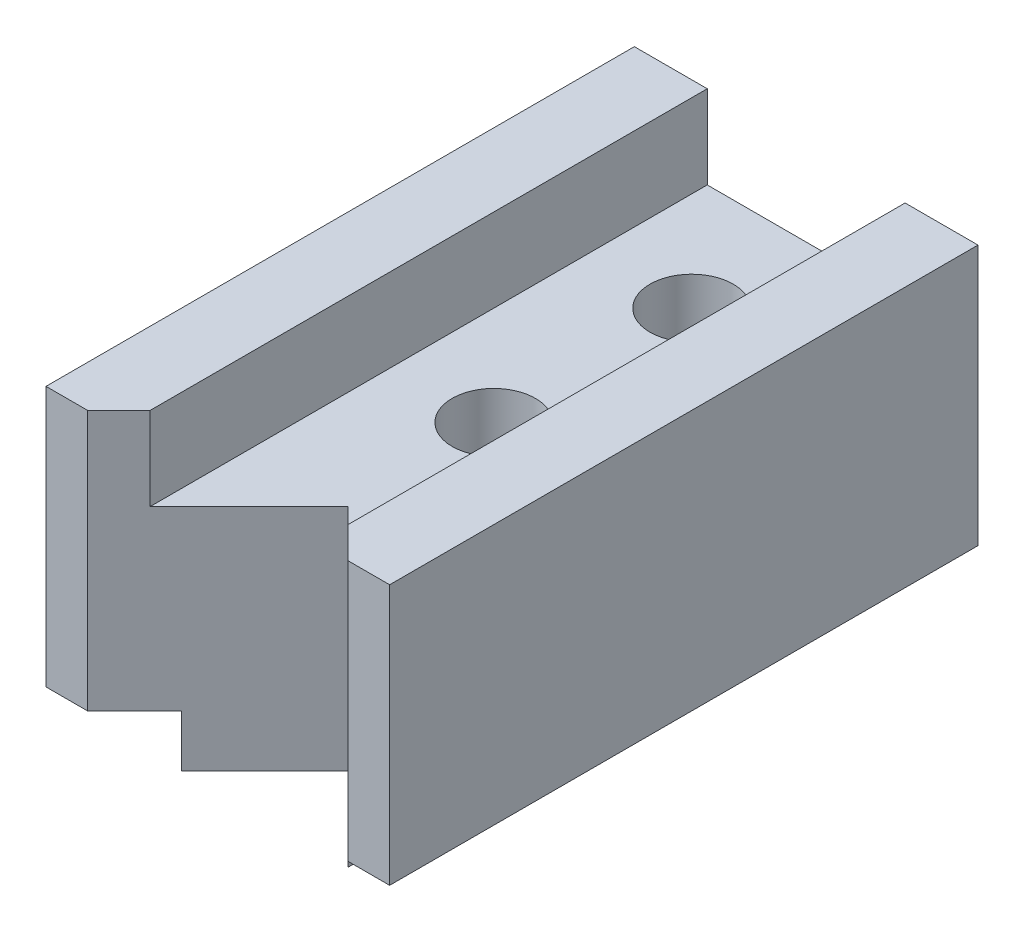
ISO-10303-21;
HEADER;
FILE_DESCRIPTION(('STEP AP214'),'2;1');
FILE_NAME('part.step','',(''),(''),'','','');
FILE_SCHEMA(('AUTOMOTIVE_DESIGN { 1 0 10303 214 1 1 1 1 }'));
ENDSEC;
DATA;
#1=APPLICATION_CONTEXT('core data for automotive mechanical design processes');
#2=APPLICATION_PROTOCOL_DEFINITION('international standard','automotive_design',2000,#1);
#3=PRODUCT_CONTEXT('',#1,'mechanical');
#4=PRODUCT('Part','Part','',(#3));
#5=PRODUCT_RELATED_PRODUCT_CATEGORY('part','',(#4));
#6=PRODUCT_DEFINITION_FORMATION('','',#4);
#7=PRODUCT_DEFINITION_CONTEXT('part definition',#1,'design');
#8=PRODUCT_DEFINITION('design','',#6,#7);
#9=PRODUCT_DEFINITION_SHAPE('','',#8);
#10=(LENGTH_UNIT() NAMED_UNIT(*) SI_UNIT(.MILLI.,.METRE.));
#11=(NAMED_UNIT(*) PLANE_ANGLE_UNIT() SI_UNIT($,.RADIAN.));
#12=(NAMED_UNIT(*) SI_UNIT($,.STERADIAN.) SOLID_ANGLE_UNIT());
#13=UNCERTAINTY_MEASURE_WITH_UNIT(LENGTH_MEASURE(1.E-05),#10,'distance_accuracy_value','');
#14=(GEOMETRIC_REPRESENTATION_CONTEXT(3) GLOBAL_UNCERTAINTY_ASSIGNED_CONTEXT((#13)) GLOBAL_UNIT_ASSIGNED_CONTEXT((#10,
#11,#12)) REPRESENTATION_CONTEXT('',''));
#15=CARTESIAN_POINT('',(0.,0.,0.));
#16=DIRECTION('',(0.,0.,1.));
#17=DIRECTION('',(1.,0.,0.));
#18=AXIS2_PLACEMENT_3D('',#15,#16,#17);
#19=CARTESIAN_POINT('',(0.,0.,56.5));
#20=DIRECTION('',(0.,0.,-1.));
#21=DIRECTION('',(-1.,0.,0.));
#22=AXIS2_PLACEMENT_3D('',#19,#20,#21);
#23=PLANE('',#22);
#24=DIRECTION('',(0.,-1.,0.));
#25=VECTOR('',#24,1.);
#26=CARTESIAN_POINT('',(8.00000000000009,179.9522506111,56.5));
#27=LINE('',#26,#25);
#28=CARTESIAN_POINT('',(8.00000000000009,50.,56.5));
#29=VERTEX_POINT('',#28);
#30=CARTESIAN_POINT('',(8.00000000000009,0.,56.5));
#31=VERTEX_POINT('',#30);
#32=EDGE_CURVE('E11',#29,#31,#27,.T.);
#33=ORIENTED_EDGE('',*,*,#32,.F.);
#34=DIRECTION('',(-1.,0.,0.));
#35=VECTOR('',#34,1.);
#36=CARTESIAN_POINT('',(0.,50.,56.5));
#37=LINE('',#36,#35);
#38=CARTESIAN_POINT('',(0.,50.,56.5));
#39=VERTEX_POINT('',#38);
#40=EDGE_CURVE('E180',#29,#39,#37,.T.);
#41=ORIENTED_EDGE('',*,*,#40,.T.);
#42=DIRECTION('',(0.,-1.,0.));
#43=VECTOR('',#42,1.);
#44=CARTESIAN_POINT('',(0.,0.,56.5));
#45=LINE('',#44,#43);
#46=CARTESIAN_POINT('',(0.,0.,56.5));
#47=VERTEX_POINT('',#46);
#48=EDGE_CURVE('E64',#39,#47,#45,.T.);
#49=ORIENTED_EDGE('',*,*,#48,.T.);
#50=DIRECTION('',(1.,0.,0.));
#51=VECTOR('',#50,1.);
#52=CARTESIAN_POINT('',(17.,0.,56.5));
#53=LINE('',#52,#51);
#54=EDGE_CURVE('E220',#47,#31,#53,.T.);
#55=ORIENTED_EDGE('',*,*,#54,.T.);
#56=EDGE_LOOP('',(#33,#41,#49,#55));
#57=FACE_BOUND('',#56,.T.);
#58=ADVANCED_FACE('F39',(#57),#23,.F.);
#59=CARTESIAN_POINT('',(17.,0.,56.5));
#60=DIRECTION('',(0.,1.,0.));
#61=DIRECTION('',(0.,0.,1.));
#62=AXIS2_PLACEMENT_3D('',#59,#60,#61);
#63=PLANE('',#62);
#64=DIRECTION('',(0.,0.,-1.));
#65=VECTOR('',#64,1.);
#66=CARTESIAN_POINT('',(17.,0.,56.5));
#67=LINE('',#66,#65);
#68=CARTESIAN_POINT('',(17.,0.,47.5000000000001));
#69=VERTEX_POINT('',#68);
#70=CARTESIAN_POINT('',(17.,0.,-56.5));
#71=VERTEX_POINT('',#70);
#72=EDGE_CURVE('E43',#69,#71,#67,.T.);
#73=ORIENTED_EDGE('',*,*,#72,.F.);
#74=DIRECTION('',(-0.707106781186546,0.,0.707106781186549));
#75=VECTOR('',#74,1.);
#76=CARTESIAN_POINT('',(12.5,0.,52.));
#77=LINE('',#76,#75);
#78=EDGE_CURVE('E419',#69,#31,#77,.T.);
#79=ORIENTED_EDGE('',*,*,#78,.T.);
#80=ORIENTED_EDGE('',*,*,#54,.F.);
#81=DIRECTION('',(0.,0.,-1.));
#82=VECTOR('',#81,1.);
#83=CARTESIAN_POINT('',(0.,0.,56.5));
#84=LINE('',#83,#82);
#85=CARTESIAN_POINT('',(0.,0.,-56.5));
#86=VERTEX_POINT('',#85);
#87=EDGE_CURVE('E183',#47,#86,#84,.T.);
#88=ORIENTED_EDGE('',*,*,#87,.T.);
#89=DIRECTION('',(1.,0.,0.));
#90=VECTOR('',#89,1.);
#91=CARTESIAN_POINT('',(17.,0.,-56.5));
#92=LINE('',#91,#90);
#93=EDGE_CURVE('E186',#86,#71,#92,.T.);
#94=ORIENTED_EDGE('',*,*,#93,.T.);
#95=EDGE_LOOP('',(#73,#79,#80,#88,#94));
#96=FACE_BOUND('',#95,.T.);
#97=ADVANCED_FACE('F41',(#96),#63,.F.);
#98=CARTESIAN_POINT('',(17.,-10.,56.5));
#99=DIRECTION('',(1.,0.,0.));
#100=DIRECTION('',(0.,0.,-1.));
#101=AXIS2_PLACEMENT_3D('',#98,#99,#100);
#102=PLANE('',#101);
#103=DIRECTION('',(0.,0.,-1.));
#104=VECTOR('',#103,1.);
#105=CARTESIAN_POINT('',(17.,-10.,56.5));
#106=LINE('',#105,#104);
#107=CARTESIAN_POINT('',(17.,-10.,47.5000000000001));
#108=VERTEX_POINT('',#107);
#109=CARTESIAN_POINT('',(17.,-10.,-56.5));
#110=VERTEX_POINT('',#109);
#111=EDGE_CURVE('E237',#108,#110,#106,.T.);
#112=ORIENTED_EDGE('',*,*,#111,.F.);
#113=DIRECTION('',(0.,1.,0.));
#114=VECTOR('',#113,1.);
#115=CARTESIAN_POINT('',(17.,-10.,47.5000000000001));
#116=LINE('',#115,#114);
#117=EDGE_CURVE('E249',#108,#69,#116,.T.);
#118=ORIENTED_EDGE('',*,*,#117,.T.);
#119=ORIENTED_EDGE('',*,*,#72,.T.);
#120=DIRECTION('',(0.,-1.,0.));
#121=VECTOR('',#120,1.);
#122=CARTESIAN_POINT('',(17.,-10.,-56.5));
#123=LINE('',#122,#121);
#124=EDGE_CURVE('E188',#71,#110,#123,.T.);
#125=ORIENTED_EDGE('',*,*,#124,.T.);
#126=EDGE_LOOP('',(#112,#118,#119,#125));
#127=FACE_BOUND('',#126,.T.);
#128=ADVANCED_FACE('F243',(#127),#102,.F.);
#129=CARTESIAN_POINT('',(49.,-10.,56.5));
#130=DIRECTION('',(0.,1.,0.));
#131=DIRECTION('',(-1.,0.,0.));
#132=AXIS2_PLACEMENT_3D('',#129,#130,#131);
#133=PLANE('',#132);
#134=CARTESIAN_POINT('',(33.,-10.,-34.5));
#135=DIRECTION('',(0.,1.,0.));
#136=DIRECTION('',(0.,0.,1.));
#137=AXIS2_PLACEMENT_3D('',#134,#135,#136);
#138=CIRCLE('',#137,8.);
#139=CARTESIAN_POINT('',(33.,-10.,-26.5));
#140=VERTEX_POINT('',#139);
#141=EDGE_CURVE('E189',#140,#140,#138,.T.);
#142=ORIENTED_EDGE('',*,*,#141,.T.);
#143=EDGE_LOOP('',(#142));
#144=FACE_BOUND('',#143,.T.);
#145=CARTESIAN_POINT('',(33.,-10.,3.5));
#146=DIRECTION('',(0.,1.,0.));
#147=DIRECTION('',(0.,0.,1.));
#148=AXIS2_PLACEMENT_3D('',#145,#146,#147);
#149=CIRCLE('',#148,8.);
#150=CARTESIAN_POINT('',(33.,-10.,11.5));
#151=VERTEX_POINT('',#150);
#152=EDGE_CURVE('E424',#151,#151,#149,.T.);
#153=ORIENTED_EDGE('',*,*,#152,.T.);
#154=EDGE_LOOP('',(#153));
#155=FACE_BOUND('',#154,.T.);
#156=DIRECTION('',(-0.707106781186547,0.,-0.707106781186549));
#157=VECTOR('',#156,1.);
#158=CARTESIAN_POINT('',(53.5,-10.,52.));
#159=LINE('',#158,#157);
#160=CARTESIAN_POINT('',(49.,-10.,47.5));
#161=VERTEX_POINT('',#160);
#162=CARTESIAN_POINT('',(33.,-10.,31.5));
#163=VERTEX_POINT('',#162);
#164=EDGE_CURVE('E287',#161,#163,#159,.T.);
#165=ORIENTED_EDGE('',*,*,#164,.T.);
#166=DIRECTION('',(-0.707106781186546,0.,0.707106781186549));
#167=VECTOR('',#166,1.);
#168=CARTESIAN_POINT('',(28.5,-10.,36.));
#169=LINE('',#168,#167);
#170=EDGE_CURVE('E426',#163,#108,#169,.T.);
#171=ORIENTED_EDGE('',*,*,#170,.T.);
#172=ORIENTED_EDGE('',*,*,#111,.T.);
#173=DIRECTION('',(1.,0.,0.));
#174=VECTOR('',#173,1.);
#175=CARTESIAN_POINT('',(49.,-10.,-56.5));
#176=LINE('',#175,#174);
#177=CARTESIAN_POINT('',(49.,-10.,-56.5));
#178=VERTEX_POINT('',#177);
#179=EDGE_CURVE('E195',#110,#178,#176,.T.);
#180=ORIENTED_EDGE('',*,*,#179,.T.);
#181=DIRECTION('',(0.,0.,-1.));
#182=VECTOR('',#181,1.);
#183=CARTESIAN_POINT('',(49.,-10.,56.5));
#184=LINE('',#183,#182);
#185=EDGE_CURVE('E232',#161,#178,#184,.T.);
#186=ORIENTED_EDGE('',*,*,#185,.F.);
#187=EDGE_LOOP('',(#165,#171,#172,#180,#186));
#188=FACE_BOUND('',#187,.T.);
#189=ADVANCED_FACE('F288',(#144,#155,#188),#133,.F.);
#190=CARTESIAN_POINT('',(49.,0.,56.5));
#191=DIRECTION('',(-1.,0.,0.));
#192=DIRECTION('',(0.,0.,1.));
#193=AXIS2_PLACEMENT_3D('',#190,#191,#192);
#194=PLANE('',#193);
#195=DIRECTION('',(0.,0.,-1.));
#196=VECTOR('',#195,1.);
#197=CARTESIAN_POINT('',(49.,0.,56.5));
#198=LINE('',#197,#196);
#199=CARTESIAN_POINT('',(49.,0.,47.5));
#200=VERTEX_POINT('',#199);
#201=CARTESIAN_POINT('',(49.,0.,-56.5));
#202=VERTEX_POINT('',#201);
#203=EDGE_CURVE('E235',#200,#202,#198,.T.);
#204=ORIENTED_EDGE('',*,*,#203,.F.);
#205=DIRECTION('',(0.,-1.,0.));
#206=VECTOR('',#205,1.);
#207=CARTESIAN_POINT('',(49.,0.,47.5));
#208=LINE('',#207,#206);
#209=EDGE_CURVE('E286',#200,#161,#208,.T.);
#210=ORIENTED_EDGE('',*,*,#209,.T.);
#211=ORIENTED_EDGE('',*,*,#185,.T.);
#212=DIRECTION('',(0.,1.,0.));
#213=VECTOR('',#212,1.);
#214=CARTESIAN_POINT('',(49.,0.,-56.5));
#215=LINE('',#214,#213);
#216=EDGE_CURVE('E198',#178,#202,#215,.T.);
#217=ORIENTED_EDGE('',*,*,#216,.T.);
#218=EDGE_LOOP('',(#204,#210,#211,#217));
#219=FACE_BOUND('',#218,.T.);
#220=ADVANCED_FACE('F284',(#219),#194,.F.);
#221=CARTESIAN_POINT('',(66.,0.,56.5));
#222=DIRECTION('',(0.,1.,0.));
#223=DIRECTION('',(0.,0.,1.));
#224=AXIS2_PLACEMENT_3D('',#221,#222,#223);
#225=PLANE('',#224);
#226=DIRECTION('',(1.,0.,0.));
#227=VECTOR('',#226,1.);
#228=CARTESIAN_POINT('',(66.,0.,56.5));
#229=LINE('',#228,#227);
#230=CARTESIAN_POINT('',(57.9999999999999,0.,56.5));
#231=VERTEX_POINT('',#230);
#232=CARTESIAN_POINT('',(66.,0.,56.5));
#233=VERTEX_POINT('',#232);
#234=EDGE_CURVE('E117',#231,#233,#229,.T.);
#235=ORIENTED_EDGE('',*,*,#234,.F.);
#236=DIRECTION('',(-0.707106781186547,0.,-0.707106781186549));
#237=VECTOR('',#236,1.);
#238=CARTESIAN_POINT('',(62.,0.,60.5));
#239=LINE('',#238,#237);
#240=EDGE_CURVE('E161',#231,#200,#239,.T.);
#241=ORIENTED_EDGE('',*,*,#240,.T.);
#242=ORIENTED_EDGE('',*,*,#203,.T.);
#243=DIRECTION('',(1.,0.,0.));
#244=VECTOR('',#243,1.);
#245=CARTESIAN_POINT('',(66.,0.,-56.5));
#246=LINE('',#245,#244);
#247=CARTESIAN_POINT('',(66.,0.,-56.5));
#248=VERTEX_POINT('',#247);
#249=EDGE_CURVE('E200',#202,#248,#246,.T.);
#250=ORIENTED_EDGE('',*,*,#249,.T.);
#251=DIRECTION('',(0.,0.,-1.));
#252=VECTOR('',#251,1.);
#253=CARTESIAN_POINT('',(66.,0.,56.5));
#254=LINE('',#253,#252);
#255=EDGE_CURVE('E229',#233,#248,#254,.T.);
#256=ORIENTED_EDGE('',*,*,#255,.F.);
#257=EDGE_LOOP('',(#235,#241,#242,#250,#256));
#258=FACE_BOUND('',#257,.T.);
#259=ADVANCED_FACE('F281',(#258),#225,.F.);
#260=CARTESIAN_POINT('',(66.,50.,56.5));
#261=DIRECTION('',(-1.,0.,0.));
#262=DIRECTION('',(0.,0.,1.));
#263=AXIS2_PLACEMENT_3D('',#260,#261,#262);
#264=PLANE('',#263);
#265=DIRECTION('',(0.,1.,0.));
#266=VECTOR('',#265,1.);
#267=CARTESIAN_POINT('',(66.,50.,-56.5));
#268=LINE('',#267,#266);
#269=CARTESIAN_POINT('',(66.,50.,-56.5));
#270=VERTEX_POINT('',#269);
#271=EDGE_CURVE('E203',#248,#270,#268,.T.);
#272=ORIENTED_EDGE('',*,*,#271,.T.);
#273=DIRECTION('',(0.,0.,-1.));
#274=VECTOR('',#273,1.);
#275=CARTESIAN_POINT('',(66.,50.,56.5));
#276=LINE('',#275,#274);
#277=CARTESIAN_POINT('',(66.,50.,56.5));
#278=VERTEX_POINT('',#277);
#279=EDGE_CURVE('E227',#278,#270,#276,.T.);
#280=ORIENTED_EDGE('',*,*,#279,.F.);
#281=DIRECTION('',(0.,1.,0.));
#282=VECTOR('',#281,1.);
#283=CARTESIAN_POINT('',(66.,50.,56.5));
#284=LINE('',#283,#282);
#285=EDGE_CURVE('E179',#233,#278,#284,.T.);
#286=ORIENTED_EDGE('',*,*,#285,.F.);
#287=ORIENTED_EDGE('',*,*,#255,.T.);
#288=EDGE_LOOP('',(#272,#280,#286,#287));
#289=FACE_BOUND('',#288,.T.);
#290=ADVANCED_FACE('F279',(#289),#264,.F.);
#291=CARTESIAN_POINT('',(52.,50.,56.5));
#292=DIRECTION('',(0.,-1.,0.));
#293=DIRECTION('',(0.,0.,-1.));
#294=AXIS2_PLACEMENT_3D('',#291,#292,#293);
#295=PLANE('',#294);
#296=DIRECTION('',(0.,0.,-1.));
#297=VECTOR('',#296,1.);
#298=CARTESIAN_POINT('',(52.,50.,56.5));
#299=LINE('',#298,#297);
#300=CARTESIAN_POINT('',(52.,50.,50.5000000000001));
#301=VERTEX_POINT('',#300);
#302=CARTESIAN_POINT('',(52.,50.,-56.5));
#303=VERTEX_POINT('',#302);
#304=EDGE_CURVE('E171',#301,#303,#299,.T.);
#305=ORIENTED_EDGE('',*,*,#304,.F.);
#306=DIRECTION('',(0.707106781186547,0.,0.707106781186549));
#307=VECTOR('',#306,1.);
#308=CARTESIAN_POINT('',(55.,50.,53.5));
#309=LINE('',#308,#307);
#310=CARTESIAN_POINT('',(57.9999999999999,50.,56.5));
#311=VERTEX_POINT('',#310);
#312=EDGE_CURVE('E158',#301,#311,#309,.T.);
#313=ORIENTED_EDGE('',*,*,#312,.T.);
#314=DIRECTION('',(-1.,0.,0.));
#315=VECTOR('',#314,1.);
#316=CARTESIAN_POINT('',(52.,50.,56.5));
#317=LINE('',#316,#315);
#318=EDGE_CURVE('E166',#278,#311,#317,.T.);
#319=ORIENTED_EDGE('',*,*,#318,.F.);
#320=ORIENTED_EDGE('',*,*,#279,.T.);
#321=DIRECTION('',(-1.,0.,0.));
#322=VECTOR('',#321,1.);
#323=CARTESIAN_POINT('',(52.,50.,-56.5));
#324=LINE('',#323,#322);
#325=EDGE_CURVE('E201',#270,#303,#324,.T.);
#326=ORIENTED_EDGE('',*,*,#325,.T.);
#327=EDGE_LOOP('',(#305,#313,#319,#320,#326));
#328=FACE_BOUND('',#327,.T.);
#329=ADVANCED_FACE('F170',(#328),#295,.F.);
#330=CARTESIAN_POINT('',(52.,34.,56.5));
#331=DIRECTION('',(1.,0.,0.));
#332=DIRECTION('',(0.,0.,-1.));
#333=AXIS2_PLACEMENT_3D('',#330,#331,#332);
#334=PLANE('',#333);
#335=DIRECTION('',(0.,0.,-1.));
#336=VECTOR('',#335,1.);
#337=CARTESIAN_POINT('',(52.,34.,56.5));
#338=LINE('',#337,#336);
#339=CARTESIAN_POINT('',(52.,34.,50.5));
#340=VERTEX_POINT('',#339);
#341=CARTESIAN_POINT('',(52.,34.,-56.5));
#342=VERTEX_POINT('',#341);
#343=EDGE_CURVE('E223',#340,#342,#338,.T.);
#344=ORIENTED_EDGE('',*,*,#343,.F.);
#345=DIRECTION('',(0.,1.,0.));
#346=VECTOR('',#345,1.);
#347=CARTESIAN_POINT('',(52.,34.,50.5000000000001));
#348=LINE('',#347,#346);
#349=EDGE_CURVE('E175',#340,#301,#348,.T.);
#350=ORIENTED_EDGE('',*,*,#349,.T.);
#351=ORIENTED_EDGE('',*,*,#304,.T.);
#352=DIRECTION('',(0.,-1.,0.));
#353=VECTOR('',#352,1.);
#354=CARTESIAN_POINT('',(52.,34.,-56.5));
#355=LINE('',#354,#353);
#356=EDGE_CURVE('E202',#303,#342,#355,.T.);
#357=ORIENTED_EDGE('',*,*,#356,.T.);
#358=EDGE_LOOP('',(#344,#350,#351,#357));
#359=FACE_BOUND('',#358,.T.);
#360=ADVANCED_FACE('F277',(#359),#334,.F.);
#361=CARTESIAN_POINT('',(14.,34.,56.5));
#362=DIRECTION('',(0.,-1.,0.));
#363=DIRECTION('',(0.,0.,-1.));
#364=AXIS2_PLACEMENT_3D('',#361,#362,#363);
#365=PLANE('',#364);
#366=CARTESIAN_POINT('',(33.,34.,-34.5));
#367=DIRECTION('',(0.,1.,0.));
#368=DIRECTION('',(0.,0.,1.));
#369=AXIS2_PLACEMENT_3D('',#366,#367,#368);
#370=CIRCLE('',#369,8.);
#371=CARTESIAN_POINT('',(33.,34.,-26.5));
#372=VERTEX_POINT('',#371);
#373=EDGE_CURVE('E431',#372,#372,#370,.T.);
#374=ORIENTED_EDGE('',*,*,#373,.F.);
#375=EDGE_LOOP('',(#374));
#376=FACE_BOUND('',#375,.T.);
#377=CARTESIAN_POINT('',(33.,34.,3.5));
#378=DIRECTION('',(0.,1.,0.));
#379=DIRECTION('',(0.,0.,1.));
#380=AXIS2_PLACEMENT_3D('',#377,#378,#379);
#381=CIRCLE('',#380,8.);
#382=CARTESIAN_POINT('',(33.,34.,11.5));
#383=VERTEX_POINT('',#382);
#384=EDGE_CURVE('E423',#383,#383,#381,.T.);
#385=ORIENTED_EDGE('',*,*,#384,.F.);
#386=EDGE_LOOP('',(#385));
#387=FACE_BOUND('',#386,.T.);
#388=DIRECTION('',(0.,0.,-1.));
#389=VECTOR('',#388,1.);
#390=CARTESIAN_POINT('',(14.,34.,56.5));
#391=LINE('',#390,#389);
#392=CARTESIAN_POINT('',(14.,34.,50.5000000000001));
#393=VERTEX_POINT('',#392);
#394=CARTESIAN_POINT('',(14.,34.,-56.5));
#395=VERTEX_POINT('',#394);
#396=EDGE_CURVE('E224',#393,#395,#391,.T.);
#397=ORIENTED_EDGE('',*,*,#396,.F.);
#398=DIRECTION('',(0.707106781186546,0.,-0.707106781186549));
#399=VECTOR('',#398,1.);
#400=CARTESIAN_POINT('',(11.,34.,53.5));
#401=LINE('',#400,#399);
#402=CARTESIAN_POINT('',(33.,34.,31.5));
#403=VERTEX_POINT('',#402);
#404=EDGE_CURVE('E441',#393,#403,#401,.T.);
#405=ORIENTED_EDGE('',*,*,#404,.T.);
#406=DIRECTION('',(0.707106781186547,0.,0.707106781186549));
#407=VECTOR('',#406,1.);
#408=CARTESIAN_POINT('',(36.,34.,34.5));
#409=LINE('',#408,#407);
#410=EDGE_CURVE('E451',#403,#340,#409,.T.);
#411=ORIENTED_EDGE('',*,*,#410,.T.);
#412=ORIENTED_EDGE('',*,*,#343,.T.);
#413=DIRECTION('',(-1.,0.,0.));
#414=VECTOR('',#413,1.);
#415=CARTESIAN_POINT('',(14.,34.,-56.5));
#416=LINE('',#415,#414);
#417=EDGE_CURVE('E208',#342,#395,#416,.T.);
#418=ORIENTED_EDGE('',*,*,#417,.T.);
#419=EDGE_LOOP('',(#397,#405,#411,#412,#418));
#420=FACE_BOUND('',#419,.T.);
#421=ADVANCED_FACE('F267',(#376,#387,#420),#365,.F.);
#422=CARTESIAN_POINT('',(14.,50.,56.5));
#423=DIRECTION('',(-1.,0.,0.));
#424=DIRECTION('',(0.,-1.,0.));
#425=AXIS2_PLACEMENT_3D('',#422,#423,#424);
#426=PLANE('',#425);
#427=DIRECTION('',(0.,0.,-1.));
#428=VECTOR('',#427,1.);
#429=CARTESIAN_POINT('',(14.,50.,56.5));
#430=LINE('',#429,#428);
#431=CARTESIAN_POINT('',(14.,50.,50.5000000000001));
#432=VERTEX_POINT('',#431);
#433=CARTESIAN_POINT('',(14.,50.,-56.5));
#434=VERTEX_POINT('',#433);
#435=EDGE_CURVE('E222',#432,#434,#430,.T.);
#436=ORIENTED_EDGE('',*,*,#435,.F.);
#437=DIRECTION('',(0.,-1.,0.));
#438=VECTOR('',#437,1.);
#439=CARTESIAN_POINT('',(14.,50.,50.5000000000001));
#440=LINE('',#439,#438);
#441=EDGE_CURVE('E57',#432,#393,#440,.T.);
#442=ORIENTED_EDGE('',*,*,#441,.T.);
#443=ORIENTED_EDGE('',*,*,#396,.T.);
#444=DIRECTION('',(0.,1.,0.));
#445=VECTOR('',#444,1.);
#446=CARTESIAN_POINT('',(14.,50.,-56.5));
#447=LINE('',#446,#445);
#448=EDGE_CURVE('E211',#395,#434,#447,.T.);
#449=ORIENTED_EDGE('',*,*,#448,.T.);
#450=EDGE_LOOP('',(#436,#442,#443,#449));
#451=FACE_BOUND('',#450,.T.);
#452=ADVANCED_FACE('F264',(#451),#426,.F.);
#453=CARTESIAN_POINT('',(0.,50.,56.5));
#454=DIRECTION('',(0.,-1.,0.));
#455=DIRECTION('',(0.,0.,-1.));
#456=AXIS2_PLACEMENT_3D('',#453,#454,#455);
#457=PLANE('',#456);
#458=ORIENTED_EDGE('',*,*,#40,.F.);
#459=DIRECTION('',(0.707106781186546,0.,-0.707106781186549));
#460=VECTOR('',#459,1.);
#461=CARTESIAN_POINT('',(4.00000000000006,50.,60.5));
#462=LINE('',#461,#460);
#463=EDGE_CURVE('E263',#29,#432,#462,.T.);
#464=ORIENTED_EDGE('',*,*,#463,.T.);
#465=ORIENTED_EDGE('',*,*,#435,.T.);
#466=DIRECTION('',(-1.,0.,0.));
#467=VECTOR('',#466,1.);
#468=CARTESIAN_POINT('',(0.,50.,-56.5));
#469=LINE('',#468,#467);
#470=CARTESIAN_POINT('',(0.,50.,-56.5));
#471=VERTEX_POINT('',#470);
#472=EDGE_CURVE('E212',#434,#471,#469,.T.);
#473=ORIENTED_EDGE('',*,*,#472,.T.);
#474=DIRECTION('',(0.,0.,-1.));
#475=VECTOR('',#474,1.);
#476=CARTESIAN_POINT('',(0.,50.,56.5));
#477=LINE('',#476,#475);
#478=EDGE_CURVE('E218',#39,#471,#477,.T.);
#479=ORIENTED_EDGE('',*,*,#478,.F.);
#480=EDGE_LOOP('',(#458,#464,#465,#473,#479));
#481=FACE_BOUND('',#480,.T.);
#482=ADVANCED_FACE('F261',(#481),#457,.F.);
#483=CARTESIAN_POINT('',(0.,0.,56.5));
#484=DIRECTION('',(1.,0.,0.));
#485=DIRECTION('',(0.,0.,-1.));
#486=AXIS2_PLACEMENT_3D('',#483,#484,#485);
#487=PLANE('',#486);
#488=DIRECTION('',(0.,-1.,0.));
#489=VECTOR('',#488,1.);
#490=CARTESIAN_POINT('',(0.,0.,-56.5));
#491=LINE('',#490,#489);
#492=EDGE_CURVE('E109',#471,#86,#491,.T.);
#493=ORIENTED_EDGE('',*,*,#492,.T.);
#494=ORIENTED_EDGE('',*,*,#87,.F.);
#495=ORIENTED_EDGE('',*,*,#48,.F.);
#496=ORIENTED_EDGE('',*,*,#478,.T.);
#497=EDGE_LOOP('',(#493,#494,#495,#496));
#498=FACE_BOUND('',#497,.T.);
#499=ADVANCED_FACE('F255',(#498),#487,.F.);
#500=ORIENTED_EDGE('',*,*,#318,.T.);
#501=DIRECTION('',(0.,-1.,0.));
#502=VECTOR('',#501,1.);
#503=CARTESIAN_POINT('',(57.9999999999999,179.9522506111,56.5));
#504=LINE('',#503,#502);
#505=EDGE_CURVE('E48',#311,#231,#504,.T.);
#506=ORIENTED_EDGE('',*,*,#505,.T.);
#507=ORIENTED_EDGE('',*,*,#234,.T.);
#508=ORIENTED_EDGE('',*,*,#285,.T.);
#509=EDGE_LOOP('',(#500,#506,#507,#508));
#510=FACE_BOUND('',#509,.T.);
#511=ADVANCED_FACE('F173',(#510),#23,.F.);
#512=CARTESIAN_POINT('',(0.,0.,-56.5));
#513=DIRECTION('',(0.,0.,-1.));
#514=DIRECTION('',(-1.,0.,0.));
#515=AXIS2_PLACEMENT_3D('',#512,#513,#514);
#516=PLANE('',#515);
#517=ORIENTED_EDGE('',*,*,#93,.F.);
#518=ORIENTED_EDGE('',*,*,#492,.F.);
#519=ORIENTED_EDGE('',*,*,#472,.F.);
#520=ORIENTED_EDGE('',*,*,#448,.F.);
#521=ORIENTED_EDGE('',*,*,#417,.F.);
#522=ORIENTED_EDGE('',*,*,#356,.F.);
#523=ORIENTED_EDGE('',*,*,#325,.F.);
#524=ORIENTED_EDGE('',*,*,#271,.F.);
#525=ORIENTED_EDGE('',*,*,#249,.F.);
#526=ORIENTED_EDGE('',*,*,#216,.F.);
#527=ORIENTED_EDGE('',*,*,#179,.F.);
#528=ORIENTED_EDGE('',*,*,#124,.F.);
#529=EDGE_LOOP('',(#517,#518,#519,#520,#521,#522,#523,#524,#525,#526,#527,#528));
#530=FACE_BOUND('',#529,.T.);
#531=ADVANCED_FACE('F253',(#530),#516,.T.);
#532=CARTESIAN_POINT('',(33.,-10.,3.5));
#533=DIRECTION('',(0.,1.,0.));
#534=DIRECTION('',(0.,0.,1.));
#535=AXIS2_PLACEMENT_3D('',#532,#533,#534);
#536=CYLINDRICAL_SURFACE('',#535,8.);
#537=ORIENTED_EDGE('',*,*,#152,.F.);
#538=EDGE_LOOP('',(#537));
#539=FACE_BOUND('',#538,.T.);
#540=ORIENTED_EDGE('',*,*,#384,.T.);
#541=EDGE_LOOP('',(#540));
#542=FACE_BOUND('',#541,.T.);
#543=ADVANCED_FACE('F316',(#539,#542),#536,.F.);
#544=CARTESIAN_POINT('',(33.,-10.,-34.5));
#545=DIRECTION('',(0.,1.,0.));
#546=DIRECTION('',(0.,0.,1.));
#547=AXIS2_PLACEMENT_3D('',#544,#545,#546);
#548=CYLINDRICAL_SURFACE('',#547,8.);
#549=ORIENTED_EDGE('',*,*,#141,.F.);
#550=EDGE_LOOP('',(#549));
#551=FACE_BOUND('',#550,.T.);
#552=ORIENTED_EDGE('',*,*,#373,.T.);
#553=EDGE_LOOP('',(#552));
#554=FACE_BOUND('',#553,.T.);
#555=ADVANCED_FACE('F386',(#551,#554),#548,.F.);
#556=CARTESIAN_POINT('',(8.00000000000009,179.9522506111,56.5));
#557=DIRECTION('',(-0.707106781186549,0.,-0.707106781186546));
#558=DIRECTION('',(-0.707106781186546,0.,0.707106781186549));
#559=AXIS2_PLACEMENT_3D('',#556,#557,#558);
#560=PLANE('',#559);
#561=ORIENTED_EDGE('',*,*,#78,.F.);
#562=ORIENTED_EDGE('',*,*,#117,.F.);
#563=ORIENTED_EDGE('',*,*,#170,.F.);
#564=DIRECTION('',(0.,-1.,0.));
#565=VECTOR('',#564,1.);
#566=CARTESIAN_POINT('',(33.,179.9522506111,31.5));
#567=LINE('',#566,#565);
#568=EDGE_CURVE('E455',#403,#163,#567,.T.);
#569=ORIENTED_EDGE('',*,*,#568,.F.);
#570=ORIENTED_EDGE('',*,*,#404,.F.);
#571=ORIENTED_EDGE('',*,*,#441,.F.);
#572=ORIENTED_EDGE('',*,*,#463,.F.);
#573=ORIENTED_EDGE('',*,*,#32,.T.);
#574=EDGE_LOOP('',(#561,#562,#563,#569,#570,#571,#572,#573));
#575=FACE_BOUND('',#574,.T.);
#576=ADVANCED_FACE('F399',(#575),#560,.F.);
#577=CARTESIAN_POINT('',(33.,179.9522506111,31.5));
#578=DIRECTION('',(0.707106781186549,0.,-0.707106781186547));
#579=DIRECTION('',(-0.707106781186547,0.,-0.707106781186549));
#580=AXIS2_PLACEMENT_3D('',#577,#578,#579);
#581=PLANE('',#580);
#582=ORIENTED_EDGE('',*,*,#164,.F.);
#583=ORIENTED_EDGE('',*,*,#209,.F.);
#584=ORIENTED_EDGE('',*,*,#240,.F.);
#585=ORIENTED_EDGE('',*,*,#505,.F.);
#586=ORIENTED_EDGE('',*,*,#312,.F.);
#587=ORIENTED_EDGE('',*,*,#349,.F.);
#588=ORIENTED_EDGE('',*,*,#410,.F.);
#589=ORIENTED_EDGE('',*,*,#568,.T.);
#590=EDGE_LOOP('',(#582,#583,#584,#585,#586,#587,#588,#589));
#591=FACE_BOUND('',#590,.T.);
#592=ADVANCED_FACE('F160',(#591),#581,.F.);
#593=CLOSED_SHELL('',(#58,#97,#128,#189,#220,#259,#290,#329,#360,#421,#452,#482,#499,#511,#531,
#543,#555,#576,#592));
#594=MANIFOLD_SOLID_BREP('B2',#593);
#595=ADVANCED_BREP_SHAPE_REPRESENTATION('',(#18,#594),#14);
#596=SHAPE_DEFINITION_REPRESENTATION(#9,#595);
ENDSEC;
END-ISO-10303-21;
